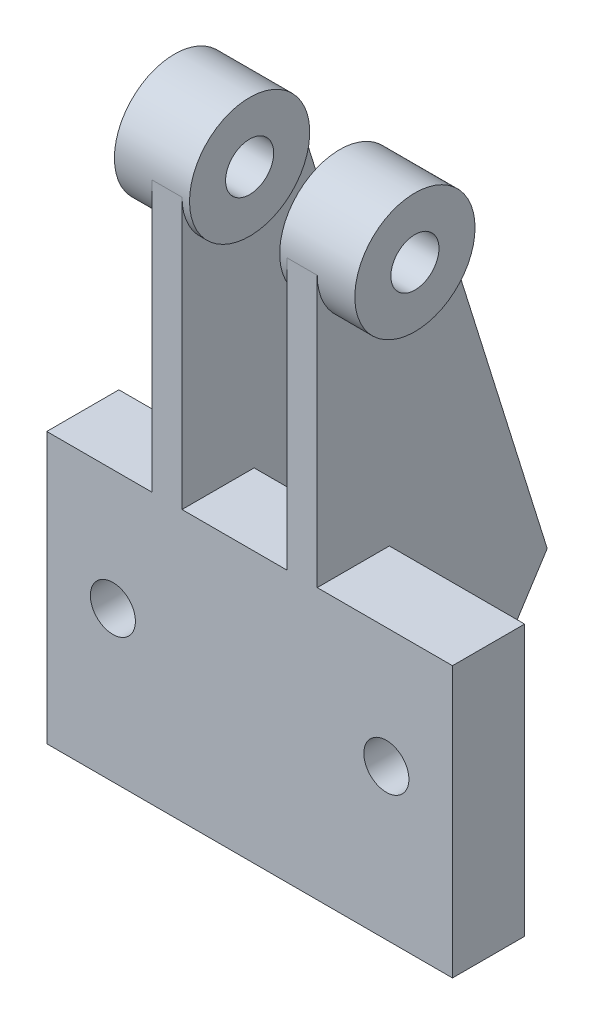
ISO-10303-21;
HEADER;
FILE_DESCRIPTION(('STEP AP214'),'2;1');
FILE_NAME('part.step','',(''),(''),'','','');
FILE_SCHEMA(('AUTOMOTIVE_DESIGN { 1 0 10303 214 1 1 1 1 }'));
ENDSEC;
DATA;
#1=APPLICATION_CONTEXT('core data for automotive mechanical design processes');
#2=APPLICATION_PROTOCOL_DEFINITION('international standard','automotive_design',2000,#1);
#3=PRODUCT_CONTEXT('',#1,'mechanical');
#4=PRODUCT('Part','Part','',(#3));
#5=PRODUCT_RELATED_PRODUCT_CATEGORY('part','',(#4));
#6=PRODUCT_DEFINITION_FORMATION('','',#4);
#7=PRODUCT_DEFINITION_CONTEXT('part definition',#1,'design');
#8=PRODUCT_DEFINITION('design','',#6,#7);
#9=PRODUCT_DEFINITION_SHAPE('','',#8);
#10=(LENGTH_UNIT() NAMED_UNIT(*) SI_UNIT(.MILLI.,.METRE.));
#11=(NAMED_UNIT(*) PLANE_ANGLE_UNIT() SI_UNIT($,.RADIAN.));
#12=(NAMED_UNIT(*) SI_UNIT($,.STERADIAN.) SOLID_ANGLE_UNIT());
#13=UNCERTAINTY_MEASURE_WITH_UNIT(LENGTH_MEASURE(1.E-05),#10,'distance_accuracy_value','');
#14=(GEOMETRIC_REPRESENTATION_CONTEXT(3) GLOBAL_UNCERTAINTY_ASSIGNED_CONTEXT((#13)) GLOBAL_UNIT_ASSIGNED_CONTEXT((#10,
#11,#12)) REPRESENTATION_CONTEXT('',''));
#15=CARTESIAN_POINT('',(0.,0.,0.));
#16=DIRECTION('',(0.,0.,1.));
#17=DIRECTION('',(1.,0.,0.));
#18=AXIS2_PLACEMENT_3D('',#15,#16,#17);
#19=CARTESIAN_POINT('',(0.,90.,-24.));
#20=DIRECTION('',(0.,1.,0.));
#21=DIRECTION('',(0.,0.,1.));
#22=AXIS2_PLACEMENT_3D('',#19,#20,#21);
#23=PLANE('',#22);
#24=DIRECTION('',(-1.,0.,0.));
#25=VECTOR('',#24,1.);
#26=CARTESIAN_POINT('',(0.,90.,-24.));
#27=LINE('',#26,#25);
#28=CARTESIAN_POINT('',(80.,90.,-24.));
#29=VERTEX_POINT('',#28);
#30=CARTESIAN_POINT('',(45.,90.,-24.));
#31=VERTEX_POINT('',#30);
#32=EDGE_CURVE('E272',#29,#31,#27,.T.);
#33=ORIENTED_EDGE('',*,*,#32,.T.);
#34=DIRECTION('',(0.,0.,1.));
#35=VECTOR('',#34,1.);
#36=CARTESIAN_POINT('',(45.,90.,0.));
#37=LINE('',#36,#35);
#38=CARTESIAN_POINT('',(45.,90.,0.));
#39=VERTEX_POINT('',#38);
#40=EDGE_CURVE('E194',#31,#39,#37,.T.);
#41=ORIENTED_EDGE('',*,*,#40,.T.);
#42=DIRECTION('',(-1.,0.,0.));
#43=VECTOR('',#42,1.);
#44=CARTESIAN_POINT('',(0.,90.,0.));
#45=LINE('',#44,#43);
#46=CARTESIAN_POINT('',(80.,90.,0.));
#47=VERTEX_POINT('',#46);
#48=EDGE_CURVE('E287',#47,#39,#45,.T.);
#49=ORIENTED_EDGE('',*,*,#48,.F.);
#50=DIRECTION('',(0.,0.,-1.));
#51=VECTOR('',#50,1.);
#52=CARTESIAN_POINT('',(80.,90.,0.));
#53=LINE('',#52,#51);
#54=EDGE_CURVE('E212',#47,#29,#53,.T.);
#55=ORIENTED_EDGE('',*,*,#54,.T.);
#56=EDGE_LOOP('',(#33,#41,#49,#55));
#57=FACE_BOUND('',#56,.T.);
#58=ADVANCED_FACE('F39',(#57),#23,.T.);
#59=CARTESIAN_POINT('',(0.,0.,-24.));
#60=DIRECTION('',(0.,0.,-1.));
#61=DIRECTION('',(-1.,0.,0.));
#62=AXIS2_PLACEMENT_3D('',#59,#60,#61);
#63=PLANE('',#62);
#64=DIRECTION('',(1.,0.,0.));
#65=VECTOR('',#64,1.);
#66=CARTESIAN_POINT('',(135.,0.,-24.));
#67=LINE('',#66,#65);
#68=CARTESIAN_POINT('',(45.,0.,-24.));
#69=VERTEX_POINT('',#68);
#70=CARTESIAN_POINT('',(80.,0.,-24.));
#71=VERTEX_POINT('',#70);
#72=EDGE_CURVE('E262',#69,#71,#67,.T.);
#73=ORIENTED_EDGE('',*,*,#72,.F.);
#74=DIRECTION('',(0.,1.,0.));
#75=VECTOR('',#74,1.);
#76=CARTESIAN_POINT('',(45.,90.,-24.));
#77=LINE('',#76,#75);
#78=EDGE_CURVE('E332',#69,#31,#77,.T.);
#79=ORIENTED_EDGE('',*,*,#78,.T.);
#80=ORIENTED_EDGE('',*,*,#32,.F.);
#81=DIRECTION('',(0.,-1.,0.));
#82=VECTOR('',#81,1.);
#83=CARTESIAN_POINT('',(80.,90.,-24.));
#84=LINE('',#83,#82);
#85=EDGE_CURVE('E220',#29,#71,#84,.T.);
#86=ORIENTED_EDGE('',*,*,#85,.T.);
#87=EDGE_LOOP('',(#73,#79,#80,#86));
#88=FACE_BOUND('',#87,.T.);
#89=ADVANCED_FACE('F344',(#88),#63,.T.);
#90=DIRECTION('',(0.,0.,1.));
#91=VECTOR('',#90,1.);
#92=CARTESIAN_POINT('',(35.,90.,0.));
#93=LINE('',#92,#91);
#94=CARTESIAN_POINT('',(35.,90.,-24.));
#95=VERTEX_POINT('',#94);
#96=CARTESIAN_POINT('',(35.,90.,0.));
#97=VERTEX_POINT('',#96);
#98=EDGE_CURVE('E320',#95,#97,#93,.T.);
#99=ORIENTED_EDGE('',*,*,#98,.F.);
#100=CARTESIAN_POINT('',(0.,90.,-24.));
#101=VERTEX_POINT('',#100);
#102=EDGE_CURVE('E268',#95,#101,#27,.T.);
#103=ORIENTED_EDGE('',*,*,#102,.T.);
#104=DIRECTION('',(0.,0.,1.));
#105=VECTOR('',#104,1.);
#106=CARTESIAN_POINT('',(0.,90.,-24.));
#107=LINE('',#106,#105);
#108=CARTESIAN_POINT('',(0.,90.,0.));
#109=VERTEX_POINT('',#108);
#110=EDGE_CURVE('E48',#101,#109,#107,.T.);
#111=ORIENTED_EDGE('',*,*,#110,.T.);
#112=EDGE_CURVE('E284',#97,#109,#45,.T.);
#113=ORIENTED_EDGE('',*,*,#112,.F.);
#114=EDGE_LOOP('',(#99,#103,#111,#113));
#115=FACE_BOUND('',#114,.T.);
#116=ADVANCED_FACE('F341',(#115),#23,.T.);
#117=CARTESIAN_POINT('',(22.,50.,-24.));
#118=DIRECTION('',(0.,0.,-1.));
#119=DIRECTION('',(-1.,0.,0.));
#120=AXIS2_PLACEMENT_3D('',#117,#118,#119);
#121=CIRCLE('',#120,7.5);
#122=CARTESIAN_POINT('',(14.5,50.,-24.));
#123=VERTEX_POINT('',#122);
#124=EDGE_CURVE('E604',#123,#123,#121,.T.);
#125=ORIENTED_EDGE('',*,*,#124,.F.);
#126=EDGE_LOOP('',(#125));
#127=FACE_BOUND('',#126,.T.);
#128=DIRECTION('',(0.,1.,0.));
#129=VECTOR('',#128,1.);
#130=CARTESIAN_POINT('',(35.,90.,-24.));
#131=LINE('',#130,#129);
#132=CARTESIAN_POINT('',(35.,0.,-24.));
#133=VERTEX_POINT('',#132);
#134=EDGE_CURVE('E199',#133,#95,#131,.T.);
#135=ORIENTED_EDGE('',*,*,#134,.F.);
#136=CARTESIAN_POINT('',(0.,0.,-24.));
#137=VERTEX_POINT('',#136);
#138=EDGE_CURVE('E257',#137,#133,#67,.T.);
#139=ORIENTED_EDGE('',*,*,#138,.F.);
#140=DIRECTION('',(0.,-1.,0.));
#141=VECTOR('',#140,1.);
#142=CARTESIAN_POINT('',(0.,0.,-24.));
#143=LINE('',#142,#141);
#144=EDGE_CURVE('E275',#101,#137,#143,.T.);
#145=ORIENTED_EDGE('',*,*,#144,.F.);
#146=ORIENTED_EDGE('',*,*,#102,.F.);
#147=EDGE_LOOP('',(#135,#139,#145,#146));
#148=FACE_BOUND('',#147,.T.);
#149=ADVANCED_FACE('F311',(#127,#148),#63,.T.);
#150=CARTESIAN_POINT('',(135.,0.,-24.));
#151=DIRECTION('',(0.,-1.,0.));
#152=DIRECTION('',(1.,0.,0.));
#153=AXIS2_PLACEMENT_3D('',#150,#151,#152);
#154=PLANE('',#153);
#155=DIRECTION('',(1.,0.,0.));
#156=VECTOR('',#155,1.);
#157=CARTESIAN_POINT('',(135.,0.,0.));
#158=LINE('',#157,#156);
#159=CARTESIAN_POINT('',(0.,0.,0.));
#160=VERTEX_POINT('',#159);
#161=CARTESIAN_POINT('',(135.,0.,0.));
#162=VERTEX_POINT('',#161);
#163=EDGE_CURVE('E251',#160,#162,#158,.T.);
#164=ORIENTED_EDGE('',*,*,#163,.F.);
#165=DIRECTION('',(0.,0.,1.));
#166=VECTOR('',#165,1.);
#167=CARTESIAN_POINT('',(0.,0.,-24.));
#168=LINE('',#167,#166);
#169=EDGE_CURVE('E11',#137,#160,#168,.T.);
#170=ORIENTED_EDGE('',*,*,#169,.F.);
#171=ORIENTED_EDGE('',*,*,#138,.T.);
#172=DIRECTION('',(0.,0.,1.));
#173=VECTOR('',#172,1.);
#174=CARTESIAN_POINT('',(35.,0.,-24.));
#175=LINE('',#174,#173);
#176=CARTESIAN_POINT('',(35.,0.,-36.));
#177=VERTEX_POINT('',#176);
#178=EDGE_CURVE('E204',#177,#133,#175,.T.);
#179=ORIENTED_EDGE('',*,*,#178,.F.);
#180=DIRECTION('',(1.,0.,0.));
#181=VECTOR('',#180,1.);
#182=CARTESIAN_POINT('',(35.,0.,-36.));
#183=LINE('',#182,#181);
#184=CARTESIAN_POINT('',(45.,0.,-36.));
#185=VERTEX_POINT('',#184);
#186=EDGE_CURVE('E203',#177,#185,#183,.T.);
#187=ORIENTED_EDGE('',*,*,#186,.T.);
#188=DIRECTION('',(0.,0.,1.));
#189=VECTOR('',#188,1.);
#190=CARTESIAN_POINT('',(45.,0.,-24.));
#191=LINE('',#190,#189);
#192=EDGE_CURVE('E196',#185,#69,#191,.T.);
#193=ORIENTED_EDGE('',*,*,#192,.T.);
#194=ORIENTED_EDGE('',*,*,#72,.T.);
#195=DIRECTION('',(0.,0.,-1.));
#196=VECTOR('',#195,1.);
#197=CARTESIAN_POINT('',(80.,0.,-24.));
#198=LINE('',#197,#196);
#199=CARTESIAN_POINT('',(80.,0.,-36.));
#200=VERTEX_POINT('',#199);
#201=EDGE_CURVE('E222',#71,#200,#198,.T.);
#202=ORIENTED_EDGE('',*,*,#201,.T.);
#203=DIRECTION('',(1.,0.,0.));
#204=VECTOR('',#203,1.);
#205=CARTESIAN_POINT('',(80.,0.,-36.));
#206=LINE('',#205,#204);
#207=CARTESIAN_POINT('',(90.,0.,-36.));
#208=VERTEX_POINT('',#207);
#209=EDGE_CURVE('E234',#200,#208,#206,.T.);
#210=ORIENTED_EDGE('',*,*,#209,.T.);
#211=DIRECTION('',(0.,0.,-1.));
#212=VECTOR('',#211,1.);
#213=CARTESIAN_POINT('',(90.,0.,-24.));
#214=LINE('',#213,#212);
#215=CARTESIAN_POINT('',(90.,0.,-24.));
#216=VERTEX_POINT('',#215);
#217=EDGE_CURVE('E236',#216,#208,#214,.T.);
#218=ORIENTED_EDGE('',*,*,#217,.F.);
#219=CARTESIAN_POINT('',(135.,0.,-24.));
#220=VERTEX_POINT('',#219);
#221=EDGE_CURVE('E264',#216,#220,#67,.T.);
#222=ORIENTED_EDGE('',*,*,#221,.T.);
#223=DIRECTION('',(0.,0.,1.));
#224=VECTOR('',#223,1.);
#225=CARTESIAN_POINT('',(135.,0.,-24.));
#226=LINE('',#225,#224);
#227=EDGE_CURVE('E277',#220,#162,#226,.T.);
#228=ORIENTED_EDGE('',*,*,#227,.T.);
#229=EDGE_LOOP('',(#164,#170,#171,#179,#187,#193,#194,#202,#210,#218,#222,#228));
#230=FACE_BOUND('',#229,.T.);
#231=ADVANCED_FACE('F41',(#230),#154,.T.);
#232=CARTESIAN_POINT('',(0.,0.,-24.));
#233=DIRECTION('',(-1.,0.,0.));
#234=DIRECTION('',(0.,0.,1.));
#235=AXIS2_PLACEMENT_3D('',#232,#233,#234);
#236=PLANE('',#235);
#237=DIRECTION('',(0.,-1.,0.));
#238=VECTOR('',#237,1.);
#239=CARTESIAN_POINT('',(0.,0.,0.));
#240=LINE('',#239,#238);
#241=EDGE_CURVE('E286',#109,#160,#240,.T.);
#242=ORIENTED_EDGE('',*,*,#241,.F.);
#243=ORIENTED_EDGE('',*,*,#110,.F.);
#244=ORIENTED_EDGE('',*,*,#144,.T.);
#245=ORIENTED_EDGE('',*,*,#169,.T.);
#246=EDGE_LOOP('',(#242,#243,#244,#245));
#247=FACE_BOUND('',#246,.T.);
#248=ADVANCED_FACE('F307',(#247),#236,.T.);
#249=DIRECTION('',(0.,0.,-1.));
#250=VECTOR('',#249,1.);
#251=CARTESIAN_POINT('',(90.,90.,0.));
#252=LINE('',#251,#250);
#253=CARTESIAN_POINT('',(90.,90.,0.));
#254=VERTEX_POINT('',#253);
#255=CARTESIAN_POINT('',(90.,90.,-24.));
#256=VERTEX_POINT('',#255);
#257=EDGE_CURVE('E211',#254,#256,#252,.T.);
#258=ORIENTED_EDGE('',*,*,#257,.F.);
#259=CARTESIAN_POINT('',(135.,90.,0.));
#260=VERTEX_POINT('',#259);
#261=EDGE_CURVE('E285',#260,#254,#45,.T.);
#262=ORIENTED_EDGE('',*,*,#261,.F.);
#263=DIRECTION('',(0.,0.,1.));
#264=VECTOR('',#263,1.);
#265=CARTESIAN_POINT('',(135.,90.,-24.));
#266=LINE('',#265,#264);
#267=CARTESIAN_POINT('',(135.,90.,-24.));
#268=VERTEX_POINT('',#267);
#269=EDGE_CURVE('E295',#268,#260,#266,.T.);
#270=ORIENTED_EDGE('',*,*,#269,.F.);
#271=EDGE_CURVE('E267',#268,#256,#27,.T.);
#272=ORIENTED_EDGE('',*,*,#271,.T.);
#273=EDGE_LOOP('',(#258,#262,#270,#272));
#274=FACE_BOUND('',#273,.T.);
#275=ADVANCED_FACE('F345',(#274),#23,.T.);
#276=CARTESIAN_POINT('',(135.,90.,-24.));
#277=DIRECTION('',(1.,0.,0.));
#278=DIRECTION('',(0.,0.,-1.));
#279=AXIS2_PLACEMENT_3D('',#276,#277,#278);
#280=PLANE('',#279);
#281=DIRECTION('',(0.,1.,0.));
#282=VECTOR('',#281,1.);
#283=CARTESIAN_POINT('',(135.,90.,0.));
#284=LINE('',#283,#282);
#285=EDGE_CURVE('E276',#162,#260,#284,.T.);
#286=ORIENTED_EDGE('',*,*,#285,.F.);
#287=ORIENTED_EDGE('',*,*,#227,.F.);
#288=DIRECTION('',(0.,1.,0.));
#289=VECTOR('',#288,1.);
#290=CARTESIAN_POINT('',(135.,90.,-24.));
#291=LINE('',#290,#289);
#292=EDGE_CURVE('E263',#220,#268,#291,.T.);
#293=ORIENTED_EDGE('',*,*,#292,.T.);
#294=ORIENTED_EDGE('',*,*,#269,.T.);
#295=EDGE_LOOP('',(#286,#287,#293,#294));
#296=FACE_BOUND('',#295,.T.);
#297=ADVANCED_FACE('F298',(#296),#280,.T.);
#298=CARTESIAN_POINT('',(113.,50.,-24.));
#299=DIRECTION('',(0.,0.,-1.));
#300=DIRECTION('',(-1.,0.,0.));
#301=AXIS2_PLACEMENT_3D('',#298,#299,#300);
#302=CIRCLE('',#301,7.50000000000001);
#303=CARTESIAN_POINT('',(105.5,50.,-24.));
#304=VERTEX_POINT('',#303);
#305=EDGE_CURVE('E597',#304,#304,#302,.T.);
#306=ORIENTED_EDGE('',*,*,#305,.F.);
#307=EDGE_LOOP('',(#306));
#308=FACE_BOUND('',#307,.T.);
#309=DIRECTION('',(0.,-1.,0.));
#310=VECTOR('',#309,1.);
#311=CARTESIAN_POINT('',(90.,90.,-24.));
#312=LINE('',#311,#310);
#313=EDGE_CURVE('E235',#256,#216,#312,.T.);
#314=ORIENTED_EDGE('',*,*,#313,.F.);
#315=ORIENTED_EDGE('',*,*,#271,.F.);
#316=ORIENTED_EDGE('',*,*,#292,.F.);
#317=ORIENTED_EDGE('',*,*,#221,.F.);
#318=EDGE_LOOP('',(#314,#315,#316,#317));
#319=FACE_BOUND('',#318,.T.);
#320=ADVANCED_FACE('F355',(#308,#319),#63,.T.);
#321=CARTESIAN_POINT('',(0.,0.,0.));
#322=DIRECTION('',(0.,0.,-1.));
#323=DIRECTION('',(-1.,0.,0.));
#324=AXIS2_PLACEMENT_3D('',#321,#322,#323);
#325=PLANE('',#324);
#326=CARTESIAN_POINT('',(113.,50.,0.));
#327=DIRECTION('',(0.,0.,-1.));
#328=DIRECTION('',(-1.,0.,0.));
#329=AXIS2_PLACEMENT_3D('',#326,#327,#328);
#330=CIRCLE('',#329,7.50000000000001);
#331=CARTESIAN_POINT('',(105.5,50.,0.));
#332=VERTEX_POINT('',#331);
#333=EDGE_CURVE('E596',#332,#332,#330,.T.);
#334=ORIENTED_EDGE('',*,*,#333,.T.);
#335=EDGE_LOOP('',(#334));
#336=FACE_BOUND('',#335,.T.);
#337=CARTESIAN_POINT('',(22.,50.,0.));
#338=DIRECTION('',(0.,0.,-1.));
#339=DIRECTION('',(-1.,0.,0.));
#340=AXIS2_PLACEMENT_3D('',#337,#338,#339);
#341=CIRCLE('',#340,7.5);
#342=CARTESIAN_POINT('',(14.5,50.,0.));
#343=VERTEX_POINT('',#342);
#344=EDGE_CURVE('E599',#343,#343,#341,.T.);
#345=ORIENTED_EDGE('',*,*,#344,.T.);
#346=EDGE_LOOP('',(#345));
#347=FACE_BOUND('',#346,.T.);
#348=ORIENTED_EDGE('',*,*,#163,.T.);
#349=ORIENTED_EDGE('',*,*,#285,.T.);
#350=ORIENTED_EDGE('',*,*,#261,.T.);
#351=DIRECTION('',(0.,-1.,0.));
#352=VECTOR('',#351,1.);
#353=CARTESIAN_POINT('',(90.,90.,0.));
#354=LINE('',#353,#352);
#355=CARTESIAN_POINT('',(90.,180.,0.));
#356=VERTEX_POINT('',#355);
#357=EDGE_CURVE('E217',#356,#254,#354,.T.);
#358=ORIENTED_EDGE('',*,*,#357,.F.);
#359=DIRECTION('',(1.,0.,0.));
#360=VECTOR('',#359,1.);
#361=CARTESIAN_POINT('',(80.,180.,0.));
#362=LINE('',#361,#360);
#363=CARTESIAN_POINT('',(80.,180.,0.));
#364=VERTEX_POINT('',#363);
#365=EDGE_CURVE('E253',#364,#356,#362,.T.);
#366=ORIENTED_EDGE('',*,*,#365,.F.);
#367=DIRECTION('',(0.,-1.,0.));
#368=VECTOR('',#367,1.);
#369=CARTESIAN_POINT('',(80.,90.,0.));
#370=LINE('',#369,#368);
#371=EDGE_CURVE('E65',#364,#47,#370,.T.);
#372=ORIENTED_EDGE('',*,*,#371,.T.);
#373=ORIENTED_EDGE('',*,*,#48,.T.);
#374=DIRECTION('',(0.,1.,0.));
#375=VECTOR('',#374,1.);
#376=CARTESIAN_POINT('',(45.,180.,0.));
#377=LINE('',#376,#375);
#378=CARTESIAN_POINT('',(45.,180.,0.));
#379=VERTEX_POINT('',#378);
#380=EDGE_CURVE('E191',#39,#379,#377,.T.);
#381=ORIENTED_EDGE('',*,*,#380,.T.);
#382=DIRECTION('',(1.,0.,0.));
#383=VECTOR('',#382,1.);
#384=CARTESIAN_POINT('',(35.,180.,0.));
#385=LINE('',#384,#383);
#386=CARTESIAN_POINT('',(35.,180.,0.));
#387=VERTEX_POINT('',#386);
#388=EDGE_CURVE('E187',#387,#379,#385,.T.);
#389=ORIENTED_EDGE('',*,*,#388,.F.);
#390=DIRECTION('',(0.,1.,0.));
#391=VECTOR('',#390,1.);
#392=CARTESIAN_POINT('',(35.,180.,0.));
#393=LINE('',#392,#391);
#394=EDGE_CURVE('E57',#97,#387,#393,.T.);
#395=ORIENTED_EDGE('',*,*,#394,.F.);
#396=ORIENTED_EDGE('',*,*,#112,.T.);
#397=ORIENTED_EDGE('',*,*,#241,.T.);
#398=EDGE_LOOP('',(#348,#349,#350,#358,#366,#372,#373,#381,#389,#395,#396,#397));
#399=FACE_BOUND('',#398,.T.);
#400=ADVANCED_FACE('F302',(#336,#347,#399),#325,.F.);
#401=CARTESIAN_POINT('',(80.,63.,-76.525653447712));
#402=DIRECTION('',(0.,0.298001107121254,-0.954565524285529));
#403=DIRECTION('',(0.,0.954565524285529,0.298001107121254));
#404=AXIS2_PLACEMENT_3D('',#401,#402,#403);
#405=PLANE('',#404);
#406=DIRECTION('',(0.,0.954565524285529,0.298001107121254));
#407=VECTOR('',#406,1.);
#408=CARTESIAN_POINT('',(90.,63.,-76.525653447712));
#409=LINE('',#408,#407);
#410=CARTESIAN_POINT('',(90.,63.,-76.525653447712));
#411=VERTEX_POINT('',#410);
#412=CARTESIAN_POINT('',(90.,180.,-40.));
#413=VERTEX_POINT('',#412);
#414=EDGE_CURVE('E241',#411,#413,#409,.T.);
#415=ORIENTED_EDGE('',*,*,#414,.F.);
#416=DIRECTION('',(1.,0.,0.));
#417=VECTOR('',#416,1.);
#418=CARTESIAN_POINT('',(80.,63.,-76.525653447712));
#419=LINE('',#418,#417);
#420=CARTESIAN_POINT('',(80.,63.,-76.525653447712));
#421=VERTEX_POINT('',#420);
#422=EDGE_CURVE('E260',#421,#411,#419,.T.);
#423=ORIENTED_EDGE('',*,*,#422,.F.);
#424=DIRECTION('',(0.,0.954565524285529,0.298001107121254));
#425=VECTOR('',#424,1.);
#426=CARTESIAN_POINT('',(80.,63.,-76.525653447712));
#427=LINE('',#426,#425);
#428=CARTESIAN_POINT('',(80.,180.,-40.));
#429=VERTEX_POINT('',#428);
#430=EDGE_CURVE('E229',#421,#429,#427,.T.);
#431=ORIENTED_EDGE('',*,*,#430,.T.);
#432=DIRECTION('',(1.,0.,0.));
#433=VECTOR('',#432,1.);
#434=CARTESIAN_POINT('',(80.,180.,-40.));
#435=LINE('',#434,#433);
#436=EDGE_CURVE('E255',#429,#413,#435,.T.);
#437=ORIENTED_EDGE('',*,*,#436,.T.);
#438=EDGE_LOOP('',(#415,#423,#431,#437));
#439=FACE_BOUND('',#438,.T.);
#440=ADVANCED_FACE('F425',(#439),#405,.T.);
#441=CARTESIAN_POINT('',(80.,0.,-36.));
#442=DIRECTION('',(0.,-0.540999888838173,-0.841022663355206));
#443=DIRECTION('',(0.,0.841022663355206,-0.540999888838173));
#444=AXIS2_PLACEMENT_3D('',#441,#442,#443);
#445=PLANE('',#444);
#446=DIRECTION('',(0.,0.841022663355206,-0.540999888838173));
#447=VECTOR('',#446,1.);
#448=CARTESIAN_POINT('',(90.,0.,-36.));
#449=LINE('',#448,#447);
#450=EDGE_CURVE('E242',#208,#411,#449,.T.);
#451=ORIENTED_EDGE('',*,*,#450,.F.);
#452=ORIENTED_EDGE('',*,*,#209,.F.);
#453=DIRECTION('',(0.,0.841022663355206,-0.540999888838173));
#454=VECTOR('',#453,1.);
#455=CARTESIAN_POINT('',(80.,0.,-36.));
#456=LINE('',#455,#454);
#457=EDGE_CURVE('E221',#200,#421,#456,.T.);
#458=ORIENTED_EDGE('',*,*,#457,.T.);
#459=ORIENTED_EDGE('',*,*,#422,.T.);
#460=EDGE_LOOP('',(#451,#452,#458,#459));
#461=FACE_BOUND('',#460,.T.);
#462=ADVANCED_FACE('F414',(#461),#445,.T.);
#463=CARTESIAN_POINT('',(80.,180.,-20.));
#464=DIRECTION('',(1.,0.,0.));
#465=DIRECTION('',(0.,0.,-1.));
#466=AXIS2_PLACEMENT_3D('',#463,#464,#465);
#467=PLANE('',#466);
#468=ORIENTED_EDGE('',*,*,#54,.F.);
#469=ORIENTED_EDGE('',*,*,#371,.F.);
#470=CARTESIAN_POINT('',(80.,180.,-20.));
#471=DIRECTION('',(-1.,0.,0.));
#472=DIRECTION('',(0.,0.,-1.));
#473=AXIS2_PLACEMENT_3D('',#470,#471,#472);
#474=CIRCLE('',#473,20.);
#475=EDGE_CURVE('E228',#429,#364,#474,.T.);
#476=ORIENTED_EDGE('',*,*,#475,.F.);
#477=ORIENTED_EDGE('',*,*,#430,.F.);
#478=ORIENTED_EDGE('',*,*,#457,.F.);
#479=ORIENTED_EDGE('',*,*,#201,.F.);
#480=ORIENTED_EDGE('',*,*,#85,.F.);
#481=EDGE_LOOP('',(#468,#469,#476,#477,#478,#479,#480));
#482=FACE_BOUND('',#481,.T.);
#483=ADVANCED_FACE('F404',(#482),#467,.F.);
#484=CARTESIAN_POINT('',(90.,180.,-20.));
#485=DIRECTION('',(1.,0.,0.));
#486=DIRECTION('',(0.,0.,-1.));
#487=AXIS2_PLACEMENT_3D('',#484,#485,#486);
#488=PLANE('',#487);
#489=ORIENTED_EDGE('',*,*,#257,.T.);
#490=ORIENTED_EDGE('',*,*,#313,.T.);
#491=ORIENTED_EDGE('',*,*,#217,.T.);
#492=ORIENTED_EDGE('',*,*,#450,.T.);
#493=ORIENTED_EDGE('',*,*,#414,.T.);
#494=CARTESIAN_POINT('',(90.,180.,-20.));
#495=DIRECTION('',(-1.,0.,0.));
#496=DIRECTION('',(0.,0.,-1.));
#497=AXIS2_PLACEMENT_3D('',#494,#495,#496);
#498=CIRCLE('',#497,20.);
#499=EDGE_CURVE('E247',#413,#356,#498,.T.);
#500=ORIENTED_EDGE('',*,*,#499,.T.);
#501=ORIENTED_EDGE('',*,*,#357,.T.);
#502=EDGE_LOOP('',(#489,#490,#491,#492,#493,#500,#501));
#503=FACE_BOUND('',#502,.T.);
#504=ADVANCED_FACE('F396',(#503),#488,.T.);
#505=CARTESIAN_POINT('',(102.5,180.,-20.));
#506=DIRECTION('',(-1.,0.,0.));
#507=DIRECTION('',(0.,0.,1.));
#508=AXIS2_PLACEMENT_3D('',#505,#506,#507);
#509=CYLINDRICAL_SURFACE('',#508,20.);
#510=CARTESIAN_POINT('',(102.5,180.,-20.));
#511=DIRECTION('',(1.,0.,0.));
#512=DIRECTION('',(0.,0.,-1.));
#513=AXIS2_PLACEMENT_3D('',#510,#511,#512);
#514=CIRCLE('',#513,20.);
#515=CARTESIAN_POINT('',(102.5,180.,-40.));
#516=VERTEX_POINT('',#515);
#517=EDGE_CURVE('E208',#516,#516,#514,.T.);
#518=ORIENTED_EDGE('',*,*,#517,.F.);
#519=EDGE_LOOP('',(#518));
#520=FACE_BOUND('',#519,.T.);
#521=CARTESIAN_POINT('',(77.5,180.,-20.));
#522=DIRECTION('',(1.,0.,0.));
#523=DIRECTION('',(0.,0.,-1.));
#524=AXIS2_PLACEMENT_3D('',#521,#522,#523);
#525=CIRCLE('',#524,20.);
#526=CARTESIAN_POINT('',(77.5,180.,-40.));
#527=VERTEX_POINT('',#526);
#528=EDGE_CURVE('E210',#527,#527,#525,.T.);
#529=ORIENTED_EDGE('',*,*,#528,.T.);
#530=EDGE_LOOP('',(#529));
#531=FACE_BOUND('',#530,.T.);
#532=ORIENTED_EDGE('',*,*,#436,.F.);
#533=ORIENTED_EDGE('',*,*,#475,.T.);
#534=ORIENTED_EDGE('',*,*,#365,.T.);
#535=ORIENTED_EDGE('',*,*,#499,.F.);
#536=EDGE_LOOP('',(#532,#533,#534,#535));
#537=FACE_BOUND('',#536,.T.);
#538=ADVANCED_FACE('F368',(#520,#531,#537),#509,.T.);
#539=CARTESIAN_POINT('',(102.5,180.,-20.));
#540=DIRECTION('',(1.,0.,0.));
#541=DIRECTION('',(0.,0.,-1.));
#542=AXIS2_PLACEMENT_3D('',#539,#540,#541);
#543=PLANE('',#542);
#544=CARTESIAN_POINT('',(102.5,180.,-20.));
#545=DIRECTION('',(1.,0.,0.));
#546=DIRECTION('',(0.,0.,-1.));
#547=AXIS2_PLACEMENT_3D('',#544,#545,#546);
#548=CIRCLE('',#547,8.);
#549=CARTESIAN_POINT('',(102.5,180.,-28.));
#550=VERTEX_POINT('',#549);
#551=EDGE_CURVE('E605',#550,#550,#548,.T.);
#552=ORIENTED_EDGE('',*,*,#551,.F.);
#553=EDGE_LOOP('',(#552));
#554=FACE_BOUND('',#553,.T.);
#555=ORIENTED_EDGE('',*,*,#517,.T.);
#556=EDGE_LOOP('',(#555));
#557=FACE_BOUND('',#556,.T.);
#558=ADVANCED_FACE('F381',(#554,#557),#543,.T.);
#559=CARTESIAN_POINT('',(77.5,180.,-20.));
#560=DIRECTION('',(1.,0.,0.));
#561=DIRECTION('',(0.,0.,-1.));
#562=AXIS2_PLACEMENT_3D('',#559,#560,#561);
#563=PLANE('',#562);
#564=CARTESIAN_POINT('',(77.5,180.,-20.));
#565=DIRECTION('',(1.,0.,0.));
#566=DIRECTION('',(0.,0.,-1.));
#567=AXIS2_PLACEMENT_3D('',#564,#565,#566);
#568=CIRCLE('',#567,8.);
#569=CARTESIAN_POINT('',(77.5,180.,-28.));
#570=VERTEX_POINT('',#569);
#571=EDGE_CURVE('E613',#570,#570,#568,.T.);
#572=ORIENTED_EDGE('',*,*,#571,.T.);
#573=EDGE_LOOP('',(#572));
#574=FACE_BOUND('',#573,.T.);
#575=ORIENTED_EDGE('',*,*,#528,.F.);
#576=EDGE_LOOP('',(#575));
#577=FACE_BOUND('',#576,.T.);
#578=ADVANCED_FACE('F380',(#574,#577),#563,.F.);
#579=CARTESIAN_POINT('',(35.,63.,-76.525653447712));
#580=DIRECTION('',(0.,-0.298001107121254,0.954565524285529));
#581=DIRECTION('',(0.,-0.954565524285529,-0.298001107121254));
#582=AXIS2_PLACEMENT_3D('',#579,#580,#581);
#583=PLANE('',#582);
#584=DIRECTION('',(0.,-0.954565524285529,-0.298001107121254));
#585=VECTOR('',#584,1.);
#586=CARTESIAN_POINT('',(45.,63.,-76.525653447712));
#587=LINE('',#586,#585);
#588=CARTESIAN_POINT('',(45.,180.,-40.));
#589=VERTEX_POINT('',#588);
#590=CARTESIAN_POINT('',(45.,63.,-76.525653447712));
#591=VERTEX_POINT('',#590);
#592=EDGE_CURVE('E167',#589,#591,#587,.T.);
#593=ORIENTED_EDGE('',*,*,#592,.T.);
#594=DIRECTION('',(1.,0.,0.));
#595=VECTOR('',#594,1.);
#596=CARTESIAN_POINT('',(35.,63.,-76.525653447712));
#597=LINE('',#596,#595);
#598=CARTESIAN_POINT('',(35.,63.,-76.525653447712));
#599=VERTEX_POINT('',#598);
#600=EDGE_CURVE('E189',#599,#591,#597,.T.);
#601=ORIENTED_EDGE('',*,*,#600,.F.);
#602=DIRECTION('',(0.,-0.954565524285529,-0.298001107121254));
#603=VECTOR('',#602,1.);
#604=CARTESIAN_POINT('',(35.,63.,-76.525653447712));
#605=LINE('',#604,#603);
#606=CARTESIAN_POINT('',(35.,180.,-40.));
#607=VERTEX_POINT('',#606);
#608=EDGE_CURVE('E181',#607,#599,#605,.T.);
#609=ORIENTED_EDGE('',*,*,#608,.F.);
#610=DIRECTION('',(1.,0.,0.));
#611=VECTOR('',#610,1.);
#612=CARTESIAN_POINT('',(35.,180.,-40.));
#613=LINE('',#612,#611);
#614=EDGE_CURVE('E182',#607,#589,#613,.T.);
#615=ORIENTED_EDGE('',*,*,#614,.T.);
#616=EDGE_LOOP('',(#593,#601,#609,#615));
#617=FACE_BOUND('',#616,.T.);
#618=ADVANCED_FACE('F185',(#617),#583,.F.);
#619=CARTESIAN_POINT('',(35.,0.,-36.));
#620=DIRECTION('',(0.,0.540999888838173,0.841022663355206));
#621=DIRECTION('',(0.,-0.841022663355206,0.540999888838173));
#622=AXIS2_PLACEMENT_3D('',#619,#620,#621);
#623=PLANE('',#622);
#624=DIRECTION('',(0.,-0.841022663355206,0.540999888838173));
#625=VECTOR('',#624,1.);
#626=CARTESIAN_POINT('',(45.,0.,-36.));
#627=LINE('',#626,#625);
#628=EDGE_CURVE('E171',#591,#185,#627,.T.);
#629=ORIENTED_EDGE('',*,*,#628,.T.);
#630=ORIENTED_EDGE('',*,*,#186,.F.);
#631=DIRECTION('',(0.,-0.841022663355206,0.540999888838173));
#632=VECTOR('',#631,1.);
#633=CARTESIAN_POINT('',(35.,0.,-36.));
#634=LINE('',#633,#632);
#635=EDGE_CURVE('E327',#599,#177,#634,.T.);
#636=ORIENTED_EDGE('',*,*,#635,.F.);
#637=ORIENTED_EDGE('',*,*,#600,.T.);
#638=EDGE_LOOP('',(#629,#630,#636,#637));
#639=FACE_BOUND('',#638,.T.);
#640=ADVANCED_FACE('F496',(#639),#623,.F.);
#641=CARTESIAN_POINT('',(35.,180.,-20.));
#642=DIRECTION('',(-1.,0.,0.));
#643=DIRECTION('',(0.,0.,1.));
#644=AXIS2_PLACEMENT_3D('',#641,#642,#643);
#645=PLANE('',#644);
#646=ORIENTED_EDGE('',*,*,#134,.T.);
#647=ORIENTED_EDGE('',*,*,#98,.T.);
#648=ORIENTED_EDGE('',*,*,#394,.T.);
#649=CARTESIAN_POINT('',(35.,180.,-20.));
#650=DIRECTION('',(1.,0.,0.));
#651=DIRECTION('',(0.,0.,1.));
#652=AXIS2_PLACEMENT_3D('',#649,#650,#651);
#653=CIRCLE('',#652,20.);
#654=EDGE_CURVE('E324',#387,#607,#653,.T.);
#655=ORIENTED_EDGE('',*,*,#654,.T.);
#656=ORIENTED_EDGE('',*,*,#608,.T.);
#657=ORIENTED_EDGE('',*,*,#635,.T.);
#658=ORIENTED_EDGE('',*,*,#178,.T.);
#659=EDGE_LOOP('',(#646,#647,#648,#655,#656,#657,#658));
#660=FACE_BOUND('',#659,.T.);
#661=ADVANCED_FACE('F336',(#660),#645,.T.);
#662=CARTESIAN_POINT('',(45.,180.,-20.));
#663=DIRECTION('',(-1.,0.,0.));
#664=DIRECTION('',(0.,0.,1.));
#665=AXIS2_PLACEMENT_3D('',#662,#663,#664);
#666=PLANE('',#665);
#667=ORIENTED_EDGE('',*,*,#78,.F.);
#668=ORIENTED_EDGE('',*,*,#192,.F.);
#669=ORIENTED_EDGE('',*,*,#628,.F.);
#670=ORIENTED_EDGE('',*,*,#592,.F.);
#671=CARTESIAN_POINT('',(45.,180.,-20.));
#672=DIRECTION('',(1.,0.,0.));
#673=DIRECTION('',(0.,0.,1.));
#674=AXIS2_PLACEMENT_3D('',#671,#672,#673);
#675=CIRCLE('',#674,20.);
#676=EDGE_CURVE('E172',#379,#589,#675,.T.);
#677=ORIENTED_EDGE('',*,*,#676,.F.);
#678=ORIENTED_EDGE('',*,*,#380,.F.);
#679=ORIENTED_EDGE('',*,*,#40,.F.);
#680=EDGE_LOOP('',(#667,#668,#669,#670,#677,#678,#679));
#681=FACE_BOUND('',#680,.T.);
#682=ADVANCED_FACE('F166',(#681),#666,.F.);
#683=CARTESIAN_POINT('',(22.5,180.,-20.));
#684=DIRECTION('',(1.,0.,0.));
#685=DIRECTION('',(0.,0.,-1.));
#686=AXIS2_PLACEMENT_3D('',#683,#684,#685);
#687=CYLINDRICAL_SURFACE('',#686,20.);
#688=ORIENTED_EDGE('',*,*,#654,.F.);
#689=ORIENTED_EDGE('',*,*,#388,.T.);
#690=ORIENTED_EDGE('',*,*,#676,.T.);
#691=ORIENTED_EDGE('',*,*,#614,.F.);
#692=EDGE_LOOP('',(#688,#689,#690,#691));
#693=FACE_BOUND('',#692,.T.);
#694=CARTESIAN_POINT('',(22.5,180.,-20.));
#695=DIRECTION('',(-1.,0.,0.));
#696=DIRECTION('',(0.,0.,1.));
#697=AXIS2_PLACEMENT_3D('',#694,#695,#696);
#698=CIRCLE('',#697,20.);
#699=CARTESIAN_POINT('',(22.5,180.,0.));
#700=VERTEX_POINT('',#699);
#701=EDGE_CURVE('E334',#700,#700,#698,.T.);
#702=ORIENTED_EDGE('',*,*,#701,.F.);
#703=EDGE_LOOP('',(#702));
#704=FACE_BOUND('',#703,.T.);
#705=CARTESIAN_POINT('',(47.5,180.,-20.));
#706=DIRECTION('',(-1.,0.,0.));
#707=DIRECTION('',(0.,0.,1.));
#708=AXIS2_PLACEMENT_3D('',#705,#706,#707);
#709=CIRCLE('',#708,20.);
#710=CARTESIAN_POINT('',(47.5,180.,0.));
#711=VERTEX_POINT('',#710);
#712=EDGE_CURVE('E321',#711,#711,#709,.T.);
#713=ORIENTED_EDGE('',*,*,#712,.T.);
#714=EDGE_LOOP('',(#713));
#715=FACE_BOUND('',#714,.T.);
#716=ADVANCED_FACE('F186',(#693,#704,#715),#687,.T.);
#717=CARTESIAN_POINT('',(22.5,180.,-20.));
#718=DIRECTION('',(-1.,0.,0.));
#719=DIRECTION('',(0.,0.,1.));
#720=AXIS2_PLACEMENT_3D('',#717,#718,#719);
#721=PLANE('',#720);
#722=CARTESIAN_POINT('',(22.5,180.,-20.));
#723=DIRECTION('',(-1.,0.,0.));
#724=DIRECTION('',(0.,0.,1.));
#725=AXIS2_PLACEMENT_3D('',#722,#723,#724);
#726=CIRCLE('',#725,8.);
#727=CARTESIAN_POINT('',(22.5,180.,-12.));
#728=VERTEX_POINT('',#727);
#729=EDGE_CURVE('E614',#728,#728,#726,.T.);
#730=ORIENTED_EDGE('',*,*,#729,.F.);
#731=EDGE_LOOP('',(#730));
#732=FACE_BOUND('',#731,.T.);
#733=ORIENTED_EDGE('',*,*,#701,.T.);
#734=EDGE_LOOP('',(#733));
#735=FACE_BOUND('',#734,.T.);
#736=ADVANCED_FACE('F531',(#732,#735),#721,.T.);
#737=CARTESIAN_POINT('',(47.5,180.,-20.));
#738=DIRECTION('',(-1.,0.,0.));
#739=DIRECTION('',(0.,0.,1.));
#740=AXIS2_PLACEMENT_3D('',#737,#738,#739);
#741=PLANE('',#740);
#742=CARTESIAN_POINT('',(47.5,180.,-20.));
#743=DIRECTION('',(-1.,0.,0.));
#744=DIRECTION('',(0.,0.,1.));
#745=AXIS2_PLACEMENT_3D('',#742,#743,#744);
#746=CIRCLE('',#745,8.);
#747=CARTESIAN_POINT('',(47.5,180.,-12.));
#748=VERTEX_POINT('',#747);
#749=EDGE_CURVE('E43',#748,#748,#746,.T.);
#750=ORIENTED_EDGE('',*,*,#749,.T.);
#751=EDGE_LOOP('',(#750));
#752=FACE_BOUND('',#751,.T.);
#753=ORIENTED_EDGE('',*,*,#712,.F.);
#754=EDGE_LOOP('',(#753));
#755=FACE_BOUND('',#754,.T.);
#756=ADVANCED_FACE('F545',(#752,#755),#741,.F.);
#757=CARTESIAN_POINT('',(0.,180.,-20.));
#758=DIRECTION('',(1.,0.,0.));
#759=DIRECTION('',(0.,0.,-1.));
#760=AXIS2_PLACEMENT_3D('',#757,#758,#759);
#761=CYLINDRICAL_SURFACE('',#760,8.);
#762=ORIENTED_EDGE('',*,*,#729,.T.);
#763=EDGE_LOOP('',(#762));
#764=FACE_BOUND('',#763,.T.);
#765=ORIENTED_EDGE('',*,*,#749,.F.);
#766=EDGE_LOOP('',(#765));
#767=FACE_BOUND('',#766,.T.);
#768=ADVANCED_FACE('F555',(#764,#767),#761,.F.);
#769=ORIENTED_EDGE('',*,*,#551,.T.);
#770=EDGE_LOOP('',(#769));
#771=FACE_BOUND('',#770,.T.);
#772=ORIENTED_EDGE('',*,*,#571,.F.);
#773=EDGE_LOOP('',(#772));
#774=FACE_BOUND('',#773,.T.);
#775=ADVANCED_FACE('F562',(#771,#774),#761,.F.);
#776=CARTESIAN_POINT('',(22.,50.,0.));
#777=DIRECTION('',(0.,0.,-1.));
#778=DIRECTION('',(-1.,0.,0.));
#779=AXIS2_PLACEMENT_3D('',#776,#777,#778);
#780=CYLINDRICAL_SURFACE('',#779,7.5);
#781=CARTESIAN_POINT('',(14.5,50.,0.));
#782=CARTESIAN_POINT('',(14.5,50.,-0.249999999999996));
#783=CARTESIAN_POINT('',(14.5,50.,-0.499999999999997));
#784=CARTESIAN_POINT('',(14.5,50.,-0.999999999999997));
#785=CARTESIAN_POINT('',(14.5,50.,-1.25));
#786=CARTESIAN_POINT('',(14.5,50.,-1.75));
#787=CARTESIAN_POINT('',(14.5,50.,-2.));
#788=CARTESIAN_POINT('',(14.5,50.,-2.5));
#789=CARTESIAN_POINT('',(14.5,50.,-2.75));
#790=CARTESIAN_POINT('',(14.5,50.,-3.25));
#791=CARTESIAN_POINT('',(14.5,50.,-3.5));
#792=CARTESIAN_POINT('',(14.5,50.,-4.));
#793=CARTESIAN_POINT('',(14.5,50.,-4.25));
#794=CARTESIAN_POINT('',(14.5,50.,-4.75));
#795=CARTESIAN_POINT('',(14.5,50.,-5.));
#796=CARTESIAN_POINT('',(14.5,50.,-5.5));
#797=CARTESIAN_POINT('',(14.5,50.,-5.75));
#798=CARTESIAN_POINT('',(14.5,50.,-6.25));
#799=CARTESIAN_POINT('',(14.5,50.,-6.5));
#800=CARTESIAN_POINT('',(14.5,50.,-7.));
#801=CARTESIAN_POINT('',(14.5,50.,-7.25));
#802=CARTESIAN_POINT('',(14.5,50.,-7.75));
#803=CARTESIAN_POINT('',(14.5,50.,-8.));
#804=CARTESIAN_POINT('',(14.5,50.,-8.5));
#805=CARTESIAN_POINT('',(14.5,50.,-8.75));
#806=CARTESIAN_POINT('',(14.5,50.,-9.25));
#807=CARTESIAN_POINT('',(14.5,50.,-9.5));
#808=CARTESIAN_POINT('',(14.5,50.,-10.));
#809=CARTESIAN_POINT('',(14.5,50.,-10.25));
#810=CARTESIAN_POINT('',(14.5,50.,-10.75));
#811=CARTESIAN_POINT('',(14.5,50.,-11.));
#812=CARTESIAN_POINT('',(14.5,50.,-11.5));
#813=CARTESIAN_POINT('',(14.5,50.,-11.75));
#814=CARTESIAN_POINT('',(14.5,50.,-12.25));
#815=CARTESIAN_POINT('',(14.5,50.,-12.5));
#816=CARTESIAN_POINT('',(14.5,50.,-13.));
#817=CARTESIAN_POINT('',(14.5,50.,-13.25));
#818=CARTESIAN_POINT('',(14.5,50.,-13.75));
#819=CARTESIAN_POINT('',(14.5,50.,-14.));
#820=CARTESIAN_POINT('',(14.5,50.,-14.5));
#821=CARTESIAN_POINT('',(14.5,50.,-14.75));
#822=CARTESIAN_POINT('',(14.5,50.,-15.25));
#823=CARTESIAN_POINT('',(14.5,50.,-15.5));
#824=CARTESIAN_POINT('',(14.5,50.,-16.));
#825=CARTESIAN_POINT('',(14.5,50.,-16.25));
#826=CARTESIAN_POINT('',(14.5,50.,-16.75));
#827=CARTESIAN_POINT('',(14.5,50.,-17.));
#828=CARTESIAN_POINT('',(14.5,50.,-17.5));
#829=CARTESIAN_POINT('',(14.5,50.,-17.75));
#830=CARTESIAN_POINT('',(14.5,50.,-18.25));
#831=CARTESIAN_POINT('',(14.5,50.,-18.5));
#832=CARTESIAN_POINT('',(14.5,50.,-19.));
#833=CARTESIAN_POINT('',(14.5,50.,-19.25));
#834=CARTESIAN_POINT('',(14.5,50.,-19.75));
#835=CARTESIAN_POINT('',(14.5,50.,-20.));
#836=CARTESIAN_POINT('',(14.5,50.,-20.5));
#837=CARTESIAN_POINT('',(14.5,50.,-20.75));
#838=CARTESIAN_POINT('',(14.5,50.,-21.25));
#839=CARTESIAN_POINT('',(14.5,50.,-21.5));
#840=CARTESIAN_POINT('',(14.5,50.,-22.));
#841=CARTESIAN_POINT('',(14.5,50.,-22.25));
#842=CARTESIAN_POINT('',(14.5,50.,-22.75));
#843=CARTESIAN_POINT('',(14.5,50.,-23.));
#844=CARTESIAN_POINT('',(14.5,50.,-23.5));
#845=CARTESIAN_POINT('',(14.5,50.,-23.75));
#846=CARTESIAN_POINT('',(14.5,50.,-24.));
#847=B_SPLINE_CURVE_WITH_KNOTS('',3,(#781,#782,#783,#784,#785,#786,#787,#788,#789,#790,#791,
#792,#793,#794,#795,#796,#797,#798,#799,#800,#801,#802,#803,#804,#805,#806,#807,#808,#809,#810,
#811,#812,#813,#814,#815,#816,#817,#818,#819,#820,#821,#822,#823,#824,#825,#826,#827,#828,#829,
#830,#831,#832,#833,#834,#835,#836,#837,#838,#839,#840,#841,#842,#843,#844,#845,#846),
.UNSPECIFIED.,.F.,.F.,(4,2,2,2,2,2,2,2,2,2,2,2,2,2,2,2,2,2,2,2,2,2,2,2,2,2,2,2,2,2,2,2,4),(0.,
0.75,1.5,2.25,3.,3.75,4.5,5.25,6.,6.75,7.5,8.25,9.,9.75,10.5,11.25,12.,12.75,13.5,14.25,15.,
15.75,16.5,17.25,18.,18.75,19.5,20.25,21.,21.75,22.5,23.25,24.),.UNSPECIFIED.);
#848=EDGE_CURVE('BSEAM574',#343,#123,#847,.T.);
#849=ORIENTED_EDGE('',*,*,#344,.F.);
#850=ORIENTED_EDGE('',*,*,#124,.T.);
#851=ORIENTED_EDGE('',*,*,#848,.T.);
#852=ORIENTED_EDGE('',*,*,#848,.F.);
#853=EDGE_LOOP('',(#849,#851,#850,#852));
#854=FACE_BOUND('',#853,.T.);
#855=ADVANCED_FACE('F574',(#854),#780,.F.);
#856=CARTESIAN_POINT('',(113.,50.,0.));
#857=DIRECTION('',(0.,0.,-1.));
#858=DIRECTION('',(-1.,0.,0.));
#859=AXIS2_PLACEMENT_3D('',#856,#857,#858);
#860=CYLINDRICAL_SURFACE('',#859,7.50000000000001);
#861=CARTESIAN_POINT('',(105.5,50.,0.));
#862=CARTESIAN_POINT('',(105.5,50.,-0.249999999999996));
#863=CARTESIAN_POINT('',(105.5,50.,-0.499999999999997));
#864=CARTESIAN_POINT('',(105.5,50.,-0.999999999999997));
#865=CARTESIAN_POINT('',(105.5,50.,-1.25));
#866=CARTESIAN_POINT('',(105.5,50.,-1.75));
#867=CARTESIAN_POINT('',(105.5,50.,-2.));
#868=CARTESIAN_POINT('',(105.5,50.,-2.5));
#869=CARTESIAN_POINT('',(105.5,50.,-2.75));
#870=CARTESIAN_POINT('',(105.5,50.,-3.25));
#871=CARTESIAN_POINT('',(105.5,50.,-3.5));
#872=CARTESIAN_POINT('',(105.5,50.,-4.));
#873=CARTESIAN_POINT('',(105.5,50.,-4.25));
#874=CARTESIAN_POINT('',(105.5,50.,-4.75));
#875=CARTESIAN_POINT('',(105.5,50.,-5.));
#876=CARTESIAN_POINT('',(105.5,50.,-5.5));
#877=CARTESIAN_POINT('',(105.5,50.,-5.75));
#878=CARTESIAN_POINT('',(105.5,50.,-6.25));
#879=CARTESIAN_POINT('',(105.5,50.,-6.5));
#880=CARTESIAN_POINT('',(105.5,50.,-7.));
#881=CARTESIAN_POINT('',(105.5,50.,-7.25));
#882=CARTESIAN_POINT('',(105.5,50.,-7.75));
#883=CARTESIAN_POINT('',(105.5,50.,-8.));
#884=CARTESIAN_POINT('',(105.5,50.,-8.5));
#885=CARTESIAN_POINT('',(105.5,50.,-8.75));
#886=CARTESIAN_POINT('',(105.5,50.,-9.25));
#887=CARTESIAN_POINT('',(105.5,50.,-9.5));
#888=CARTESIAN_POINT('',(105.5,50.,-10.));
#889=CARTESIAN_POINT('',(105.5,50.,-10.25));
#890=CARTESIAN_POINT('',(105.5,50.,-10.75));
#891=CARTESIAN_POINT('',(105.5,50.,-11.));
#892=CARTESIAN_POINT('',(105.5,50.,-11.5));
#893=CARTESIAN_POINT('',(105.5,50.,-11.75));
#894=CARTESIAN_POINT('',(105.5,50.,-12.25));
#895=CARTESIAN_POINT('',(105.5,50.,-12.5));
#896=CARTESIAN_POINT('',(105.5,50.,-13.));
#897=CARTESIAN_POINT('',(105.5,50.,-13.25));
#898=CARTESIAN_POINT('',(105.5,50.,-13.75));
#899=CARTESIAN_POINT('',(105.5,50.,-14.));
#900=CARTESIAN_POINT('',(105.5,50.,-14.5));
#901=CARTESIAN_POINT('',(105.5,50.,-14.75));
#902=CARTESIAN_POINT('',(105.5,50.,-15.25));
#903=CARTESIAN_POINT('',(105.5,50.,-15.5));
#904=CARTESIAN_POINT('',(105.5,50.,-16.));
#905=CARTESIAN_POINT('',(105.5,50.,-16.25));
#906=CARTESIAN_POINT('',(105.5,50.,-16.75));
#907=CARTESIAN_POINT('',(105.5,50.,-17.));
#908=CARTESIAN_POINT('',(105.5,50.,-17.5));
#909=CARTESIAN_POINT('',(105.5,50.,-17.75));
#910=CARTESIAN_POINT('',(105.5,50.,-18.25));
#911=CARTESIAN_POINT('',(105.5,50.,-18.5));
#912=CARTESIAN_POINT('',(105.5,50.,-19.));
#913=CARTESIAN_POINT('',(105.5,50.,-19.25));
#914=CARTESIAN_POINT('',(105.5,50.,-19.75));
#915=CARTESIAN_POINT('',(105.5,50.,-20.));
#916=CARTESIAN_POINT('',(105.5,50.,-20.5));
#917=CARTESIAN_POINT('',(105.5,50.,-20.75));
#918=CARTESIAN_POINT('',(105.5,50.,-21.25));
#919=CARTESIAN_POINT('',(105.5,50.,-21.5));
#920=CARTESIAN_POINT('',(105.5,50.,-22.));
#921=CARTESIAN_POINT('',(105.5,50.,-22.25));
#922=CARTESIAN_POINT('',(105.5,50.,-22.75));
#923=CARTESIAN_POINT('',(105.5,50.,-23.));
#924=CARTESIAN_POINT('',(105.5,50.,-23.5));
#925=CARTESIAN_POINT('',(105.5,50.,-23.75));
#926=CARTESIAN_POINT('',(105.5,50.,-24.));
#927=B_SPLINE_CURVE_WITH_KNOTS('',3,(#861,#862,#863,#864,#865,#866,#867,#868,#869,#870,#871,
#872,#873,#874,#875,#876,#877,#878,#879,#880,#881,#882,#883,#884,#885,#886,#887,#888,#889,#890,
#891,#892,#893,#894,#895,#896,#897,#898,#899,#900,#901,#902,#903,#904,#905,#906,#907,#908,#909,
#910,#911,#912,#913,#914,#915,#916,#917,#918,#919,#920,#921,#922,#923,#924,#925,#926),
.UNSPECIFIED.,.F.,.F.,(4,2,2,2,2,2,2,2,2,2,2,2,2,2,2,2,2,2,2,2,2,2,2,2,2,2,2,2,2,2,2,2,4),(0.,
0.75,1.5,2.25,3.,3.75,4.5,5.25,6.,6.75,7.5,8.25,9.,9.75,10.5,11.25,12.,12.75,13.5,14.25,15.,
15.75,16.5,17.25,18.,18.75,19.5,20.25,21.,21.75,22.5,23.25,24.),.UNSPECIFIED.);
#928=EDGE_CURVE('BSEAM580',#332,#304,#927,.T.);
#929=ORIENTED_EDGE('',*,*,#333,.F.);
#930=ORIENTED_EDGE('',*,*,#305,.T.);
#931=ORIENTED_EDGE('',*,*,#928,.T.);
#932=ORIENTED_EDGE('',*,*,#928,.F.);
#933=EDGE_LOOP('',(#929,#931,#930,#932));
#934=FACE_BOUND('',#933,.T.);
#935=ADVANCED_FACE('F580',(#934),#860,.F.);
#936=CLOSED_SHELL('',(#58,#89,#116,#149,#231,#248,#275,#297,#320,#400,#440,#462,#483,#504,#538,
#558,#578,#618,#640,#661,#682,#716,#736,#756,#768,#775,#855,#935));
#937=MANIFOLD_SOLID_BREP('B2',#936);
#938=ADVANCED_BREP_SHAPE_REPRESENTATION('',(#18,#937),#14);
#939=SHAPE_DEFINITION_REPRESENTATION(#9,#938);
ENDSEC;
END-ISO-10303-21;
